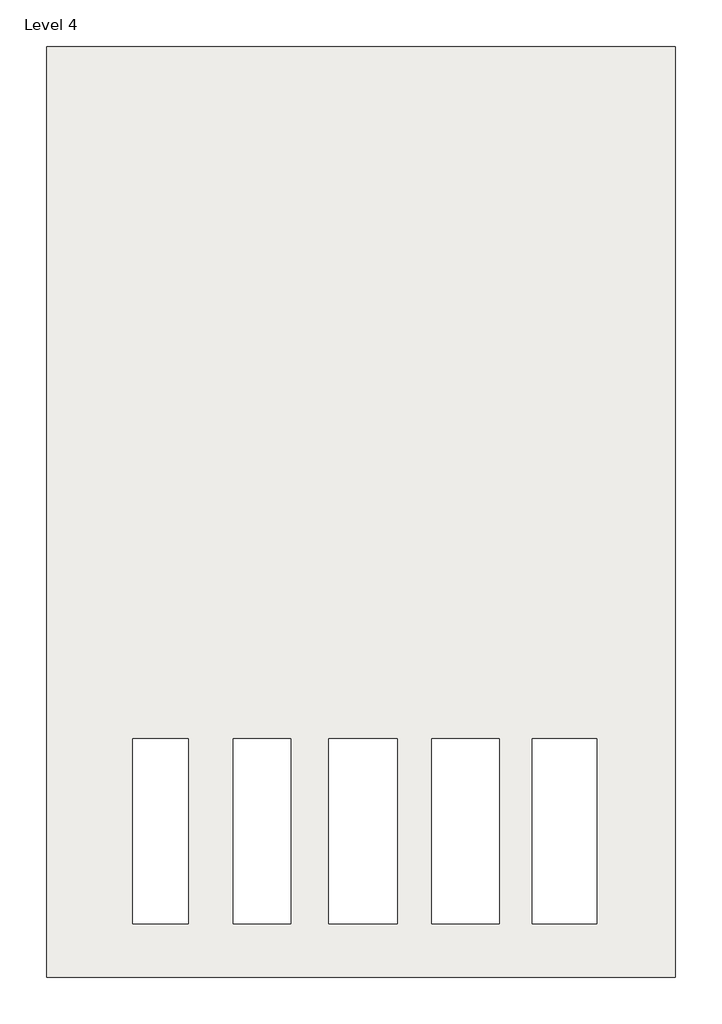
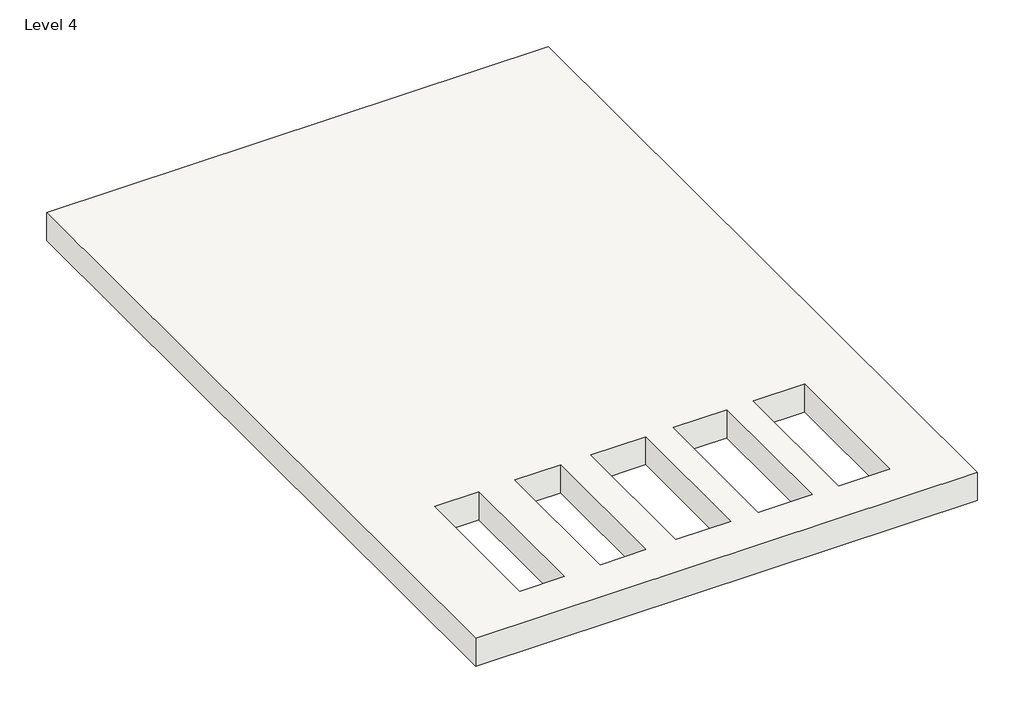
# One storey: 1 roof.
"""IFC4 building model written with IfcOpenShell, lengths in millimetres."""

from ifc_helpers import new_model, si_unit, frame, origin, place, context, project, spatial, polyline, outline, extrude, element, save

model = new_model("IFC4")

# Units and contexts
model_context = context("Model", 3, world=origin())
ifc_project = project(units=[si_unit("LENGTHUNIT", "METRE", prefix="MILLI")], contexts=[model_context])

# Site, building, storey
site = spatial("IfcSite", under=ifc_project)
building = spatial("IfcBuilding", under=site)
storey = spatial("IfcBuildingStorey", under=building, Name="Level 4", Elevation=10972.8)

# Roof
placement = place(None, origin())
element("IfcRoof", 1, ObjectType="Generic - 12\"", at=placement, inside=storey, context=model_context, shape_type="SweptSolid", body=[
    extrude(outline(polyline([(-8551.930251, 13952.073096), (-3370.330251, 13952.073096), (-3370.330251, 6281.273096), (-8551.930251, 6281.273096), (-8551.930251, 13952.073096)]), holes=[polyline([(-7383.530251, 6722.4926709), (-7383.530251, 8246.4926709), (-7840.730251, 8246.4926709), (-7840.730251, 6722.4926709), (-7383.530251, 6722.4926709)]), polyline([(-6537.8793668, 6722.4926709), (-6537.8793668, 8246.4926709), (-7012.2315451, 8246.4926709), (-7012.2315451, 6722.4926709), (-6537.8793668, 6722.4926709)]), polyline([(-5662.1522685, 6722.4926709), (-5662.1522685, 8246.4926709), (-6227.7260195, 8246.4926709), (-6227.7260195, 6722.4926709), (-5662.1522685, 6722.4926709)]), polyline([(-4822.9137992, 6722.4926709), (-4822.9137992, 8246.4926709), (-5376.930251, 8246.4926709), (-5376.930251, 6722.4926709), (-4822.9137992, 6722.4926709)]), polyline([(-4020.163959, 6722.4926709), (-4020.163959, 8246.4926709), (-4549.249081, 8246.4926709), (-4549.249081, 6722.4926709), (-4020.163959, 6722.4926709)])]), frame((0.0, 0.0, 10972.8), z_axis=(0.0, 0.0, 1.0), x_axis=(1.0, 0.0, 0.0)), (0.0, 0.0, 1.0), 304.8),
])

save(model, "model.ifc")

# Revit data of these elements
# Type "Generic - 12\""
#   Assembly Code = "B1020"
#   Layers, outside or top first: 1' - 0" no material (function 1)
# Element 1 (IfcRoof, "Generic - 12\"")
#   built-in parameter 1001705 = 37 (stored number, unit not read)
#   built-in parameter 1001710 = 33615
#   Phase Created = New Construction
#   Materials on its faces: "Default Roof"
# Materials
#   "Default Roof": colour RGB 88 101 114, transparency 0
